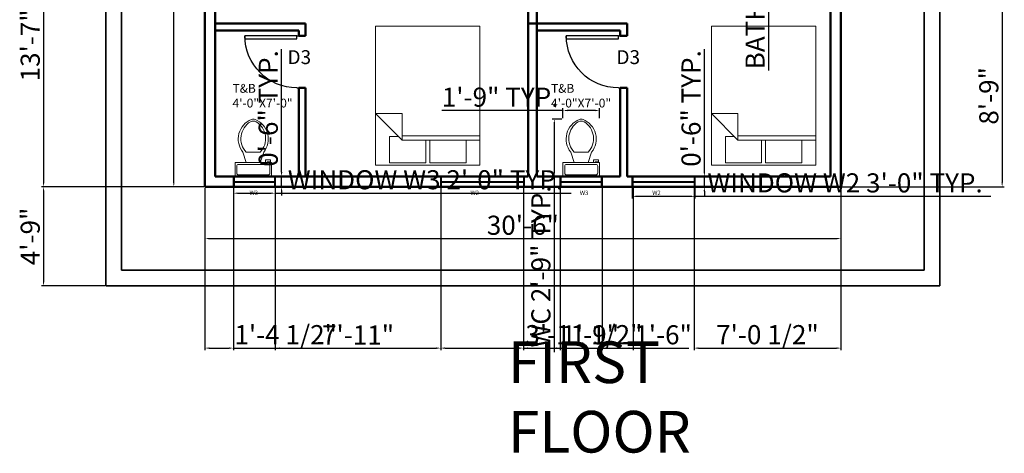
# Model space of a CAD drawing. Units: inches. Extents: x 2299 to 4423, y 1066 to 1805.
# Tile 4 of 7: x 3069 to 3636, y 1066 to 1315. Entities that reach past the tile are written whole.
import ezdxf

# ---------------------------------------------------------------- set-up
doc = ezdxf.new("R2010")
doc.units = ezdxf.units.IN
for name, color, linetype, lineweight in [('A-ANNO-DIMS', 2, 'Continuous', 18), ('A-ANNO-TEXT', 1, 'Continuous', 25), ('A-AREA-IDEN', 1, 'Continuous', 25), ('A-DOOR', 5, 'Continuous', 25), ('A-FURN', 8, 'Continuous', 18), ('A-GLAZ', 3, 'Continuous', 25), ('A-WALL', 7, 'Continuous', 50), ('C-PROP', 7, 'Continuous', 35)]:
    doc.layers.add(name, color=color, linetype=linetype, lineweight=lineweight)
doc.styles.get("Standard").update_dxf_attribs({"font": 'arial.ttf'})
doc.dimstyles.new('ISO-25', dxfattribs={"dimtxt": 11, "dimasz": 2.5, "dimexe": 1.25, "dimexo": 0.625, "dimtad": 1, "dimlunit": 4, "dimtxsty": 'Standard', "dimcen": 2.5, "dimadec": 0, "dimazin": 0, "dimtfac": 1, "dimtmove": 0, "dimatfit": 3, "dimfxl": 1, "dimarcsym": 0})

# ---------------------------------------------------------------- blocks, each defined once
blk = doc.blocks.new('*U2')
for p, q in [((0, 0), (0, -5)), ((30, 0), (30, -5))]:
    blk.add_line(p, q)
blk.add_lwpolyline([(0, 0), (0, 30), (1.75, 30), (1.75, 0)], close=True)
blk.add_arc((0, 0), 30, 0, 90)
blk = doc.blocks.new('Bed - Queen')
for p, q in [((0, -80.00003), (0, 0)), ((0, 0), (59.99999, 0)), ((59.99999, 0), (59.99999, -80.00003)), ((7.99999, -1.2), (28.79998, -1.2)), ((7.99999, -14.4), (7.99999, -1.2)), ((28.79998, -1.2), (28.79998, -14.4)), ((31.19999, -1.2), (51.99999, -1.2)), ((31.19999, -14.4), (31.19999, -1.2)), ((51.99999, -1.2), (51.99999, -16.4)), ((0, -14.4), (44.8, -14.4)), ((44.8, -16.8), (0, -16.8)), ((59.99999, -29.6), (44.8, -14.4)), ((44.8, -14.4), (44.8, -29.6)), ((51.99999, -16.4), (46.79936, -16.4)), ((44.8, -29.6), (59.99999, -29.6)), ((59.99999, -80.00003), (0, -80.00003))]:
    blk.add_line(p, q)
blk = doc.blocks.new('Toilet - top')
for p, q in [((9.5, -6), (9.5, -2)), ((-10, -8.5), (-8, -8.5)), ((-10, -9.5), (-10, -8.5)), ((-7, -9.5), (-10, -9.5)), ((-8, -8.5), (-8, -8)), ((-7, -8), (-7, -9.5)), ((-4, -8), (-6, -14)), ((4, -8), (6, -14)), ((4, -14), (-4, -14))]:
    blk.add_line(p, q)
blk.add_lwpolyline([(10.5, -8), (10.5, 0), (-10.5, 0), (-10.5, -8)], close=True)
for points in [[(-9.5, -2), (-9.5, -6)], [(8.5, -1), (-8.5, -1)], [(-8.5, -7), (8.5, -7)]]:
    blk.add_lwpolyline(points)
for centre, radius, start, end in [((-8.62, -1.88), 0.884, 81.8699, 188.1301), ((8.62, -1.88), 0.884, 351.8699, 98.1301), ((-8.62, -6.12), 0.884, 171.8699, 278.1301), ((8.62, -6.12), 0.884, 261.8699, 8.1301), ((3.52, -21.58), 12.17, 141.4691, 247.9714), ((4.2, -21.82), 11.33, 136.3677, 238.9468), ((-3.52, -21.58), 12.17, 292.0284, 38.5307), ((-4.2, -21.82), 11.33, 301.053, 43.6321), ((0, -27.88), 4, 245.7318, 294.2682), ((0, -29), 4, 254.8605, 285.1395)]:
    blk.add_arc(centre, radius, start, end)
blk = doc.blocks.new('*D24')
at = {"layer": 'A-ANNO-DIMS', "color": 0, "lineweight": -2, "transparency": 16777216}
for p, q in [((3175.75, 1218.32), (3175.75, 1187.97)), ((3541.75, 1218.32), (3541.75, 1187.97)), ((3178.25, 1189.22), (3539.25, 1189.22))]:
    blk.add_line(p, q, dxfattribs=at)
at = {"layer": 'A-ANNO-DIMS', "color": 0, "transparency": 16777216}
for points in [[(3178.25, 1189.63), (3178.25, 1188.8), (3175.75, 1189.22)], [(3539.25, 1189.63), (3539.25, 1188.8), (3541.75, 1189.22)]]:
    blk.add_solid(points, dxfattribs=at)
at = {"layer": 'Defpoints', "color": 0, "transparency": 16777216}
for p in [(3175.75, 1218.95), (3541.75, 1218.95), (3541.75, 1189.22)]:
    blk.add_point(p, dxfattribs=at)
at = {"layer": 'A-ANNO-DIMS', "color": 0, "transparency": 16777216, "insert": (3358.75, 1195.46), "char_height": 11, "attachment_point": 5}
blk.add_mtext('30\'-6"', dxfattribs=at)
blk = doc.blocks.new('*D25')
at = {"layer": 'A-ANNO-DIMS', "color": 0, "lineweight": -2, "transparency": 16777216}
for p, q in [((3175.12, 1680.95), (3156.64, 1680.95)), ((3157.89, 1221.45), (3157.89, 1678.45)), ((3175.12, 1218.95), (3156.64, 1218.95))]:
    blk.add_line(p, q, dxfattribs=at)
at = {"layer": 'A-ANNO-DIMS', "color": 0, "transparency": 16777216}
for points in [[(3157.47, 1678.45), (3158.3, 1678.45), (3157.89, 1680.95)], [(3157.47, 1221.45), (3158.3, 1221.45), (3157.89, 1218.95)]]:
    blk.add_solid(points, dxfattribs=at)
at = {"layer": 'Defpoints', "color": 0, "transparency": 16777216}
for p in [(3157.89, 1680.95), (3175.75, 1680.95), (3175.75, 1218.95)]:
    blk.add_point(p, dxfattribs=at)
at = {"layer": 'A-ANNO-DIMS', "color": 0, "transparency": 16777216, "insert": (3151.64, 1449.95), "char_height": 11, "attachment_point": 5, "rotation": 90}
blk.add_mtext('38\'-6"', dxfattribs=at)
blk = doc.blocks.new('WIN-1200')
for p, q in [((0, 0), (0, 48.07)), ((0, 48.07), (6, 48.07)), ((0, 47.57), (6, 47.57)), ((2.8, 47.57), (2.8, 0.5)), ((3.2, 47.57), (3.2, 0.5)), ((6, 48.07), (6, 0)), ((6, 0.5), (0, 0.5)), ((6, 0), (0, 0))]:
    blk.add_line(p, q)
blk = doc.blocks.new('WIN-600')
for p, q in [((0, 6), (24.07, 6)), ((0, 0), (0, 6)), ((0.5, 0), (0.5, 6)), ((23.57, 6), (23.57, 0)), ((24.07, 6), (24.07, 0)), ((24.07, 0), (0, 0)), ((0.5, 3.2), (23.57, 3.2)), ((0.5, 2.8), (23.57, 2.8))]:
    blk.add_line(p, q)
blk = doc.blocks.new('WIN-900')
for p, q in [((0, 6), (36.07, 6)), ((0, 0), (0, 6)), ((0.5, 0), (0.5, 6)), ((35.57, 6), (35.57, 0)), ((36.07, 6), (36.07, 0)), ((36.07, 0), (0, 0)), ((0.5, 3.2), (35.57, 3.2)), ((0.5, 2.8), (35.57, 2.8))]:
    blk.add_line(p, q)
blk = doc.blocks.new('*D44')
at = {"layer": 'A-ANNO-DIMS', "color": 0, "lineweight": -2, "transparency": 16777216}
for p, q in [((3192.23, 1218.32), (3192.23, 1214.08)), ((3216.3, 1218.32), (3216.3, 1214.08)), ((3194.73, 1215.33), (3213.8, 1215.33)), ((3216.3, 1215.33), (3386.57, 1215.33))]:
    blk.add_line(p, q, dxfattribs=at)
at = {"layer": 'A-ANNO-DIMS', "color": 0, "transparency": 16777216}
for points in [[(3194.73, 1215.75), (3194.73, 1214.92), (3192.23, 1215.33)], [(3213.8, 1215.75), (3213.8, 1214.92), (3216.3, 1215.33)]]:
    blk.add_solid(points, dxfattribs=at)
at = {"layer": 'Defpoints', "color": 0, "transparency": 16777216}
for p in [(3192.23, 1218.95), (3216.3, 1218.95), (3216.3, 1215.33)]:
    blk.add_point(p, dxfattribs=at)
at = {"layer": 'A-ANNO-DIMS', "color": 0, "transparency": 16777216, "insert": (3302.69, 1221.65), "char_height": 11, "attachment_point": 5}
blk.add_mtext('WINDOW W3 2\'-0" TYP.', dxfattribs=at)
blk = doc.blocks.new('*D45')
at = {"layer": 'A-ANNO-DIMS', "color": 0, "lineweight": -2, "transparency": 16777216}
for p, q in [((3219.92, 1227.45), (3219.92, 1298.25)), ((3216.93, 1224.95), (3221.17, 1224.95)), ((3219.92, 1218.95), (3219.92, 1224.95)), ((3216.93, 1218.95), (3221.17, 1218.95)), ((3219.92, 1216.45), (3219.92, 1213.95))]:
    blk.add_line(p, q, dxfattribs=at)
at = {"layer": 'A-ANNO-DIMS', "color": 0, "transparency": 16777216}
for points in [[(3219.5, 1227.45), (3220.33, 1227.45), (3219.92, 1224.95)], [(3219.5, 1216.45), (3220.33, 1216.45), (3219.92, 1218.95)]]:
    blk.add_solid(points, dxfattribs=at)
at = {"layer": 'Defpoints', "color": 0, "transparency": 16777216}
for p in [(3216.3, 1224.95), (3219.92, 1224.95), (3216.3, 1218.95)]:
    blk.add_point(p, dxfattribs=at)
at = {"layer": 'A-ANNO-DIMS', "color": 0, "transparency": 16777216, "insert": (3213.67, 1264.1), "char_height": 11, "attachment_point": 5, "rotation": 90}
blk.add_mtext('0\'-6" TYP.', dxfattribs=at)
blk = doc.blocks.new('*D46')
at = {"layer": 'A-ANNO-DIMS', "color": 0, "lineweight": -2, "transparency": 16777216}
for p, q in [((3381.19, 1257.99), (3375.61, 1257.99)), ((3376.86, 1255.49), (3376.86, 1227.45)), ((3381.19, 1224.95), (3375.61, 1224.95)), ((3376.86, 1224.95), (3376.86, 1123.82))]:
    blk.add_line(p, q, dxfattribs=at)
at = {"layer": 'A-ANNO-DIMS', "color": 0, "transparency": 16777216}
for points in [[(3376.44, 1255.49), (3377.28, 1255.49), (3376.86, 1257.99)], [(3376.44, 1227.45), (3377.28, 1227.45), (3376.86, 1224.95)]]:
    blk.add_solid(points, dxfattribs=at)
at = {"layer": 'Defpoints', "color": 0, "transparency": 16777216}
for p in [(3381.82, 1257.99), (3376.86, 1224.95), (3381.82, 1224.95)]:
    blk.add_point(p, dxfattribs=at)
at = {"layer": 'A-ANNO-DIMS', "color": 0, "transparency": 16777216, "insert": (3370.55, 1173.13), "char_height": 11, "attachment_point": 5, "rotation": 90}
blk.add_mtext('WC 2\'-9" TYP.', dxfattribs=at)
blk = doc.blocks.new('*D47')
at = {"layer": 'A-ANNO-DIMS', "color": 0, "lineweight": -2, "transparency": 16777216}
for p, q in [((3381.82, 1258.62), (3381.82, 1264.2)), ((3402.82, 1258.62), (3402.82, 1264.2)), ((3381.82, 1262.95), (3312.05, 1262.95)), ((3400.32, 1262.95), (3384.32, 1262.95))]:
    blk.add_line(p, q, dxfattribs=at)
at = {"layer": 'A-ANNO-DIMS', "color": 0, "transparency": 16777216}
for points in [[(3384.32, 1263.37), (3384.32, 1262.53), (3381.82, 1262.95)], [(3400.32, 1263.37), (3400.32, 1262.53), (3402.82, 1262.95)]]:
    blk.add_solid(points, dxfattribs=at)
at = {"layer": 'Defpoints', "color": 0, "transparency": 16777216}
for p in [(3381.82, 1262.95), (3381.82, 1257.99), (3402.82, 1257.99)]:
    blk.add_point(p, dxfattribs=at)
at = {"layer": 'A-ANNO-DIMS', "color": 0, "transparency": 16777216, "insert": (3345.68, 1269.19), "char_height": 11, "attachment_point": 5}
blk.add_mtext('1\'-9" TYP.', dxfattribs=at)
blk = doc.blocks.new('*D50')
at = {"layer": 'A-ANNO-DIMS', "color": 0, "lineweight": -2, "transparency": 16777216}
for p, q in [((3421.72, 1218.32), (3421.72, 1212.28)), ((3457.79, 1218.32), (3457.79, 1212.28)), ((3424.22, 1213.53), (3455.29, 1213.53)), ((3457.79, 1213.53), (3628.06, 1213.53))]:
    blk.add_line(p, q, dxfattribs=at)
at = {"layer": 'A-ANNO-DIMS', "color": 0, "transparency": 16777216}
for points in [[(3424.22, 1213.95), (3424.22, 1213.12), (3421.72, 1213.53)], [(3455.29, 1213.95), (3455.29, 1213.12), (3457.79, 1213.53)]]:
    blk.add_solid(points, dxfattribs=at)
at = {"layer": 'Defpoints', "color": 0, "transparency": 16777216}
for p in [(3421.72, 1218.95), (3457.79, 1218.95), (3457.79, 1213.53)]:
    blk.add_point(p, dxfattribs=at)
at = {"layer": 'A-ANNO-DIMS', "color": 0, "transparency": 16777216, "insert": (3544.17, 1219.85), "char_height": 11, "attachment_point": 5}
blk.add_mtext('WINDOW W2 3\'-0" TYP.', dxfattribs=at)
blk = doc.blocks.new('*D51')
at = {"layer": 'A-ANNO-DIMS', "color": 0, "lineweight": -2, "transparency": 16777216}
for p, q in [((3463.2, 1227.45), (3463.2, 1298.25)), ((3458.42, 1224.95), (3464.45, 1224.95)), ((3463.2, 1218.95), (3463.2, 1224.95)), ((3458.42, 1218.95), (3464.45, 1218.95)), ((3463.2, 1216.45), (3463.2, 1213.95))]:
    blk.add_line(p, q, dxfattribs=at)
at = {"layer": 'A-ANNO-DIMS', "color": 0, "transparency": 16777216}
for points in [[(3462.79, 1227.45), (3463.62, 1227.45), (3463.2, 1224.95)], [(3462.79, 1216.45), (3463.62, 1216.45), (3463.2, 1218.95)]]:
    blk.add_solid(points, dxfattribs=at)
at = {"layer": 'Defpoints', "color": 0, "transparency": 16777216}
for p in [(3457.79, 1224.95), (3463.2, 1224.95), (3457.79, 1218.95)]:
    blk.add_point(p, dxfattribs=at)
at = {"layer": 'A-ANNO-DIMS', "color": 0, "transparency": 16777216, "insert": (3456.96, 1264.1), "char_height": 11, "attachment_point": 5, "rotation": 90}
blk.add_mtext('0\'-6" TYP.', dxfattribs=at)
blk = doc.blocks.new('*D58')
at = {"layer": 'A-ANNO-DIMS', "color": 0, "lineweight": -2, "transparency": 16777216}
for p, q in [((3506.06, 1467.99), (3498.88, 1467.99)), ((3500.13, 1465.49), (3500.13, 1426.78)), ((3506.06, 1424.28), (3498.88, 1424.28)), ((3500.13, 1424.28), (3500.13, 1285.89))]:
    blk.add_line(p, q, dxfattribs=at)
at = {"layer": 'A-ANNO-DIMS', "color": 0, "transparency": 16777216}
for points in [[(3499.71, 1465.49), (3500.55, 1465.49), (3500.13, 1467.99)], [(3499.71, 1426.78), (3500.55, 1426.78), (3500.13, 1424.28)]]:
    blk.add_solid(points, dxfattribs=at)
at = {"layer": 'Defpoints', "color": 0, "transparency": 16777216}
for p in [(3506.69, 1467.99), (3500.13, 1424.28), (3506.69, 1424.28)]:
    blk.add_point(p, dxfattribs=at)
at = {"layer": 'A-ANNO-DIMS', "color": 0, "transparency": 16777216, "insert": (3493.81, 1353.83), "char_height": 11, "attachment_point": 5, "rotation": 90}
blk.add_mtext('BATH TUB 3\'-7 1/2"', dxfattribs=at)
blk = doc.blocks.new('*D102')
at = {"layer": 'A-ANNO-DIMS', "color": 0, "lineweight": -2, "transparency": 16777216}
for p, q in [((3181.12, 1381.95), (3081.7, 1381.95)), ((3082.95, 1379.45), (3082.95, 1221.45)), ((3175.12, 1218.95), (3081.7, 1218.95))]:
    blk.add_line(p, q, dxfattribs=at)
at = {"layer": 'A-ANNO-DIMS', "color": 0, "transparency": 16777216}
for points in [[(3082.53, 1379.45), (3083.37, 1379.45), (3082.95, 1381.95)], [(3082.53, 1221.45), (3083.37, 1221.45), (3082.95, 1218.95)]]:
    blk.add_solid(points, dxfattribs=at)
at = {"layer": 'Defpoints', "color": 0, "transparency": 16777216}
for p in [(3181.75, 1381.95), (3082.95, 1218.95), (3175.75, 1218.95)]:
    blk.add_point(p, dxfattribs=at)
at = {"layer": 'A-ANNO-DIMS', "color": 0, "transparency": 16777216, "insert": (3076.7, 1300.45), "char_height": 11, "attachment_point": 5, "rotation": 90}
blk.add_mtext('13\'-7"', dxfattribs=at)
blk = doc.blocks.new('*D103')
at = {"layer": 'A-ANNO-DIMS', "color": 0, "lineweight": -2, "transparency": 16777216}
for p, q in [((3175.12, 1218.95), (3081.7, 1218.95)), ((3082.95, 1216.45), (3082.95, 1164.45)), ((3118.12, 1161.95), (3081.7, 1161.95))]:
    blk.add_line(p, q, dxfattribs=at)
at = {"layer": 'A-ANNO-DIMS', "color": 0, "transparency": 16777216}
for points in [[(3082.53, 1216.45), (3083.37, 1216.45), (3082.95, 1218.95)], [(3082.53, 1164.45), (3083.37, 1164.45), (3082.95, 1161.95)]]:
    blk.add_solid(points, dxfattribs=at)
at = {"layer": 'Defpoints', "color": 0, "transparency": 16777216}
for p in [(3175.75, 1218.95), (3082.95, 1161.95), (3118.75, 1161.95)]:
    blk.add_point(p, dxfattribs=at)
at = {"layer": 'A-ANNO-DIMS', "color": 0, "transparency": 16777216, "insert": (3076.71, 1190.45), "char_height": 11, "attachment_point": 5, "rotation": 90}
blk.add_mtext('4\'-9"', dxfattribs=at)
blk = doc.blocks.new('*D108')
at = {"layer": 'A-ANNO-DIMS', "color": 0, "lineweight": -2, "transparency": 16777216}
for p, q in [((3542.37, 1323.79), (3635.8, 1323.79)), ((3634.55, 1321.29), (3634.55, 1221.45)), ((3542.37, 1218.95), (3635.8, 1218.95))]:
    blk.add_line(p, q, dxfattribs=at)
at = {"layer": 'A-ANNO-DIMS', "color": 0, "transparency": 16777216}
for points in [[(3634.13, 1321.29), (3634.97, 1321.29), (3634.55, 1323.79)], [(3634.13, 1221.45), (3634.97, 1221.45), (3634.55, 1218.95)]]:
    blk.add_solid(points, dxfattribs=at)
at = {"layer": 'Defpoints', "color": 0, "transparency": 16777216}
for p in [(3541.75, 1323.79), (3541.75, 1218.95), (3634.55, 1218.95)]:
    blk.add_point(p, dxfattribs=at)
at = {"layer": 'A-ANNO-DIMS', "color": 0, "transparency": 16777216, "insert": (3628.31, 1271.37), "char_height": 11, "attachment_point": 5, "rotation": 90}
blk.add_mtext('8\'-9"', dxfattribs=at)
blk = doc.blocks.new('*D109')
at = {"layer": 'A-ANNO-DIMS', "color": 0, "lineweight": -2, "transparency": 16777216}
for p, q in [((3175.75, 1218.32), (3175.75, 1124.9)), ((3192.23, 1218.32), (3192.23, 1124.9)), ((3178.25, 1126.15), (3189.73, 1126.15)), ((3192.23, 1126.15), (3249.82, 1126.15))]:
    blk.add_line(p, q, dxfattribs=at)
at = {"layer": 'A-ANNO-DIMS', "color": 0, "transparency": 16777216}
for points in [[(3178.25, 1126.56), (3178.25, 1125.73), (3175.75, 1126.15)], [(3189.73, 1126.56), (3189.73, 1125.73), (3192.23, 1126.15)]]:
    blk.add_solid(points, dxfattribs=at)
at = {"layer": 'Defpoints', "color": 0, "transparency": 16777216}
for p in [(3175.75, 1218.95), (3192.23, 1218.95), (3192.23, 1126.15)]:
    blk.add_point(p, dxfattribs=at)
at = {"layer": 'A-ANNO-DIMS', "color": 0, "transparency": 16777216, "insert": (3222.28, 1132.46), "char_height": 11, "attachment_point": 5}
blk.add_mtext('1\'-4 1/2"', dxfattribs=at)
blk = doc.blocks.new('*D110')
at = {"layer": 'A-ANNO-DIMS', "color": 0, "lineweight": -2, "transparency": 16777216}
for p, q in [((3216.3, 1218.32), (3216.3, 1124.9)), ((3311.49, 1218.32), (3311.49, 1124.9)), ((3218.8, 1126.15), (3308.99, 1126.15))]:
    blk.add_line(p, q, dxfattribs=at)
at = {"layer": 'A-ANNO-DIMS', "color": 0, "transparency": 16777216}
for points in [[(3218.8, 1126.56), (3218.8, 1125.73), (3216.3, 1126.15)], [(3308.99, 1126.56), (3308.99, 1125.73), (3311.49, 1126.15)]]:
    blk.add_solid(points, dxfattribs=at)
at = {"layer": 'Defpoints', "color": 0, "transparency": 16777216}
for p in [(3216.3, 1218.95), (3311.49, 1218.95), (3311.49, 1126.15)]:
    blk.add_point(p, dxfattribs=at)
at = {"layer": 'A-ANNO-DIMS', "color": 0, "transparency": 16777216, "insert": (3263.9, 1132.29), "char_height": 11, "attachment_point": 5}
blk.add_mtext('7\'-11"', dxfattribs=at)
blk = doc.blocks.new('*D111')
at = {"layer": 'A-ANNO-DIMS', "color": 0, "lineweight": -2, "transparency": 16777216}
for p, q in [((3311.49, 1218.32), (3311.49, 1124.9)), ((3359.06, 1218.32), (3359.06, 1124.9)), ((3313.99, 1126.15), (3356.56, 1126.15)), ((3359.06, 1126.15), (3426.22, 1126.15))]:
    blk.add_line(p, q, dxfattribs=at)
at = {"layer": 'A-ANNO-DIMS', "color": 0, "transparency": 16777216}
for points in [[(3313.99, 1126.56), (3313.99, 1125.73), (3311.49, 1126.15)], [(3356.56, 1126.56), (3356.56, 1125.73), (3359.06, 1126.15)]]:
    blk.add_solid(points, dxfattribs=at)
at = {"layer": 'Defpoints', "color": 0, "transparency": 16777216}
for p in [(3311.49, 1218.95), (3359.06, 1218.95), (3359.06, 1126.15)]:
    blk.add_point(p, dxfattribs=at)
at = {"layer": 'A-ANNO-DIMS', "color": 0, "transparency": 16777216, "insert": (3393.89, 1132.46), "char_height": 11, "attachment_point": 5}
blk.add_mtext('3\'-11 1/2"', dxfattribs=at)
blk = doc.blocks.new('*D112')
at = {"layer": 'A-ANNO-DIMS', "color": 0, "lineweight": -2, "transparency": 16777216}
for p, q in [((3359.06, 1218.32), (3359.06, 1124.9)), ((3380.28, 1218.32), (3380.28, 1124.9)), ((3361.56, 1126.15), (3377.78, 1126.15)), ((3380.28, 1126.15), (3412.24, 1126.15))]:
    blk.add_line(p, q, dxfattribs=at)
at = {"layer": 'A-ANNO-DIMS', "color": 0, "transparency": 16777216}
for points in [[(3361.56, 1126.56), (3361.56, 1125.73), (3359.06, 1126.15)], [(3377.78, 1126.56), (3377.78, 1125.73), (3380.28, 1126.15)]]:
    blk.add_solid(points, dxfattribs=at)
at = {"layer": 'Defpoints', "color": 0, "transparency": 16777216}
for p in [(3359.06, 1218.95), (3380.28, 1218.95), (3380.28, 1126.15)]:
    blk.add_point(p, dxfattribs=at)
at = {"layer": 'A-ANNO-DIMS', "color": 0, "transparency": 16777216, "insert": (3397.51, 1132.39), "char_height": 11, "attachment_point": 5}
blk.add_mtext('1\'-9"', dxfattribs=at)
blk = doc.blocks.new('*D113')
at = {"layer": 'A-ANNO-DIMS', "color": 0, "lineweight": -2, "transparency": 16777216}
for p, q in [((3404.35, 1218.32), (3404.35, 1124.9)), ((3422.22, 1218.32), (3422.22, 1124.9)), ((3406.85, 1126.15), (3419.72, 1126.15)), ((3422.22, 1126.15), (3454.18, 1126.15))]:
    blk.add_line(p, q, dxfattribs=at)
at = {"layer": 'A-ANNO-DIMS', "color": 0, "transparency": 16777216}
for points in [[(3406.85, 1126.56), (3406.85, 1125.73), (3404.35, 1126.15)], [(3419.72, 1126.56), (3419.72, 1125.73), (3422.22, 1126.15)]]:
    blk.add_solid(points, dxfattribs=at)
at = {"layer": 'Defpoints', "color": 0, "transparency": 16777216}
for p in [(3404.35, 1218.95), (3422.22, 1218.95), (3422.22, 1126.15)]:
    blk.add_point(p, dxfattribs=at)
at = {"layer": 'A-ANNO-DIMS', "color": 0, "transparency": 16777216, "insert": (3439.45, 1132.39), "char_height": 11, "attachment_point": 5}
blk.add_mtext('1\'-6"', dxfattribs=at)
blk = doc.blocks.new('*D114')
at = {"layer": 'A-ANNO-DIMS', "color": 0, "lineweight": -2, "transparency": 16777216}
for p, q in [((3457.29, 1218.32), (3457.29, 1124.9)), ((3541.75, 1218.32), (3541.75, 1124.9)), ((3459.79, 1126.15), (3539.25, 1126.15))]:
    blk.add_line(p, q, dxfattribs=at)
at = {"layer": 'A-ANNO-DIMS', "color": 0, "transparency": 16777216}
for points in [[(3459.79, 1126.56), (3459.79, 1125.73), (3457.29, 1126.15)], [(3539.25, 1126.56), (3539.25, 1125.73), (3541.75, 1126.15)]]:
    blk.add_solid(points, dxfattribs=at)
at = {"layer": 'Defpoints', "color": 0, "transparency": 16777216}
for p in [(3457.29, 1218.95), (3541.75, 1218.95), (3541.75, 1126.15)]:
    blk.add_point(p, dxfattribs=at)
at = {"layer": 'A-ANNO-DIMS', "color": 0, "transparency": 16777216, "insert": (3499.52, 1132.46), "char_height": 11, "attachment_point": 5}
blk.add_mtext('7\'-0 1/2"', dxfattribs=at)

msp = doc.modelspace()

# ---------------------------------------------------------------- linework, layer by layer
at = {"layer": 'A-WALL'}
for p, q in [((3175.749, 1218.945), (3175.749, 1680.945)), ((3181.749, 1224.945), (3181.749, 1376.945)), ((3361.749, 1224.945), (3361.749, 1381.945)), ((3366.749, 1224.945), (3366.749, 1376.945)), ((3535.749, 1224.945), (3535.749, 1349.945)), ((3541.749, 1218.945), (3541.749, 1344.945)), ((3233.749, 1312.945), (3181.749, 1312.945)), ((3229.749, 1308.945), (3181.749, 1308.945)), ((3229.749, 1308.945), (3229.749, 1305.945)), ((3229.749, 1305.945), (3229.749, 1308.945)), ((3233.749, 1305.945), (3233.749, 1312.945)), ((3418.749, 1312.945), (3361.749, 1312.945)), ((3414.749, 1308.945), (3366.749, 1308.945)), ((3414.749, 1308.945), (3414.749, 1305.945)), ((3414.749, 1305.945), (3414.749, 1308.945)), ((3418.749, 1305.945), (3418.749, 1312.945)), ((3229.749, 1305.945), (3233.749, 1305.945)), ((3414.749, 1305.945), (3418.749, 1305.945)), ((3229.749, 1224.945), (3229.749, 1275.945)), ((3233.749, 1275.945), (3229.749, 1275.945)), ((3233.749, 1224.945), (3233.749, 1275.945)), ((3414.749, 1224.945), (3414.749, 1275.945)), ((3418.749, 1275.945), (3414.749, 1275.945)), ((3418.749, 1224.945), (3418.749, 1275.945)), ((3361.749, 1224.945), (3181.749, 1224.945)), ((3410.749, 1224.945), (3366.749, 1224.945)), ((3410.749, 1224.945), (3414.749, 1224.945)), ((3418.749, 1224.945), (3535.749, 1224.945)), ((3415.749, 1218.945), (3175.749, 1218.945)), ((3415.749, 1218.945), (3541.749, 1218.945))]:
    msp.add_line(p, q, dxfattribs=at)
at = {"layer": 'C-PROP'}
for p, q in [((3118.749, 1161.945), (3118.749, 1737.945)), ((3598.749, 1737.945), (3598.749, 1161.945)), ((3127.749, 1170.945), (3127.749, 1728.945)), ((3589.749, 1728.945), (3589.749, 1170.945)), ((3589.749, 1170.945), (3127.749, 1170.945)), ((3598.749, 1161.945), (3118.749, 1161.945))]:
    msp.add_line(p, q, dxfattribs=at)

# ---------------------------------------------------------------- block references
at = {"layer": 'A-DOOR', "xscale": -1, "rotation": 90}
for p in [(3228.749, 1305.945), (3413.749, 1305.945)]:
    msp.add_blockref('*U2', p, dxfattribs=at)
at = {"layer": 'A-FURN'}
for name, p, rotation in [('Bed - Queen', (3334.043, 1231.522), 179.9999999999998), ('Bed - Queen', (3527.273, 1231.522), 179.9999999999998), ('Toilet - top', (3203.62, 1224.945), 180), ('Toilet - top', (3392.317, 1224.945), 180)]:
    msp.add_blockref(name, p, dxfattribs=dict(at, rotation=rotation))
at = {"layer": 'A-GLAZ'}
for name, p in [('WIN-600', (3192.233, 1218.945)), ('WIN-600', (3380.282, 1218.945)), ('WIN-900', (3421.72, 1218.945))]:
    msp.add_blockref(name, p, dxfattribs=at)
at = {"layer": 'A-GLAZ', "rotation": 89.99999999999973}
msp.add_blockref('WIN-1200', (3359.563, 1218.945), dxfattribs=at)

# ---------------------------------------------------------------- texts
at = {"layer": 'A-ANNO-TEXT', "attachment_point": 1}
for s, width, gutter_width, insert, char_height in [('D3', 1.11117, 12.5, (3223.344, 1297.671), 8), ('D3', 1.11117, 12.5, (3412.638, 1297.671), 8), ('FIRST\\PFLOOR', 684.73543, 351.786, (3350.163, 1130.01), 24)]:
    msp.add_mtext_dynamic_manual_height_columns(s, width=width, gutter_width=gutter_width, heights=[0], dxfattribs=dict(at, insert=insert, char_height=char_height))
at = {"layer": 'A-ANNO-TEXT', "char_height": 2.5, "attachment_point": 1}
for s, insert in [('W3', (3201.458, 1216.805)), ('W2', (3328.604, 1216.805)), ('W3', (3391.551, 1216.805)), ('W2', (3433.203, 1216.805))]:
    msp.add_mtext(s, dxfattribs=dict(at, insert=insert))
at = {"layer": 'A-AREA-IDEN', "char_height": 5.07992, "attachment_point": 1}
for insert in [(3191.657, 1278.226), (3374.948, 1278.226)]:
    msp.add_mtext_dynamic_manual_height_columns('T&B\\P4\'-0"X7\'-0"', width=2.46662, gutter_width=25.4, heights=[0], dxfattribs=dict(at, insert=insert))

# ---------------------------------------------------------------- dimensions: what is measured, and where the dimension line sits
at = {"layer": 'A-ANNO-DIMS'}
for base, p1, p2, override, picture, middle in [((3157.885, 1680.945), (3175.749, 1218.945), (3175.749, 1680.945), {"dimclrd": 0, "dimclre": 0, "dimclrt": 0}, '*D25', (3151.64, 1449.945)), ((3082.949, 1218.945), (3181.749, 1381.945), (3175.749, 1218.945), {"dimdec": 1, "dimlfac": 1, "dimrnd": 0, "dimzin": 1, "dimdsep": 46, "dimlunit": 4, "dimfrac": 2}, '*D102', (3076.704, 1300.445)), ((3634.549, 1218.945), (3541.749, 1323.793), (3541.749, 1218.945), {"dimdec": 1, "dimlfac": 1, "dimrnd": 0, "dimzin": 1, "dimdsep": 46, "dimlunit": 4, "dimfrac": 2}, '*D108', (3628.308, 1271.369)), ((3082.949, 1161.945), (3175.749, 1218.945), (3118.749, 1161.945), {"dimdec": 1, "dimlfac": 1, "dimrnd": 0, "dimzin": 1, "dimdsep": 46, "dimlunit": 4, "dimfrac": 2}, '*D103', (3076.708, 1190.445))]:
    dim = msp.add_linear_dim(base=base, p1=p1, p2=p2, angle=90, dimstyle='ISO-25', override=override, dxfattribs=at)
    dim.commit()
    dim.dimension.update_dxf_attribs({"geometry": picture, "text_midpoint": middle})
for base, p1, p2, angle, text, picture, middle in [((3500.129, 1424.28), (3506.686, 1467.993), (3506.686, 1424.28), 270, 'BATH TUB <>', '*D58', (3493.812, 1353.834)), ((3219.915, 1224.945), (3216.305, 1218.945), (3216.305, 1224.945), 90, '<> TYP.', '*D45', (3213.674, 1264.096)), ((3463.202, 1224.945), (3457.791, 1218.945), (3457.791, 1224.945), 90, '<> TYP.', '*D51', (3456.961, 1264.096)), ((3381.817, 1262.949), (3402.817, 1257.992), (3381.817, 1257.992), 180, '<> TYP.', '*D47', (3345.685, 1269.19)), ((3376.861, 1224.945), (3381.817, 1257.992), (3381.817, 1224.945), 270, 'WC <> TYP.', '*D46', (3370.548, 1173.134))]:
    dim = msp.add_linear_dim(base=base, p1=p1, p2=p2, angle=angle, text=text, dimstyle='ISO-25', override={"dimdec": 1, "dimrnd": 0, "dimzin": 1, "dimlunit": 4, "dimfrac": 2}, dxfattribs=at)
    dim.commit()
    dim.dimension.update_dxf_attribs({"geometry": picture, "text_midpoint": middle})
for base, p1, p2, text, picture, middle in [((3216.305, 1215.335), (3192.234, 1218.945), (3216.305, 1218.945), 'WINDOW W3 <> TYP.', '*D44', (3302.687, 1221.655)), ((3457.791, 1213.535), (3421.72, 1218.945), (3457.791, 1218.945), 'WINDOW W2 <> TYP.', '*D50', (3544.174, 1219.855))]:
    dim = msp.add_linear_dim(base=base, p1=p1, p2=p2, text=text, dimstyle='ISO-25', override={"dimdec": 1, "dimrnd": 0, "dimzin": 1, "dimlunit": 4, "dimfrac": 2}, dxfattribs=at)
    dim.commit()
    dim.dimension.update_dxf_attribs({"geometry": picture, "text_midpoint": middle})
for base, p1, p2, override, picture, middle in [((3541.749, 1189.218), (3175.749, 1218.945), (3541.749, 1218.945), {"dimclrd": 0, "dimclre": 0, "dimclrt": 0}, '*D24', (3358.749, 1195.463)), ((3192.234, 1126.145), (3175.749, 1218.945), (3192.234, 1218.945), {"dimdec": 1, "dimlfac": 1, "dimrnd": 0, "dimzin": 1, "dimdsep": 46, "dimlunit": 4, "dimfrac": 2}, '*D109', (3222.277, 1132.458)), ((3311.492, 1126.145), (3216.305, 1218.945), (3311.492, 1218.945), {"dimdec": 1, "dimlfac": 1, "dimrnd": 0, "dimzin": 1, "dimdsep": 46, "dimlunit": 4, "dimfrac": 2}, '*D110', (3263.899, 1132.293)), ((3359.063, 1126.145), (3311.492, 1218.945), (3359.063, 1218.945), {"dimdec": 1, "dimlfac": 1, "dimrnd": 0, "dimzin": 1, "dimdsep": 46, "dimlunit": 4, "dimfrac": 2}, '*D111', (3393.894, 1132.462)), ((3380.282, 1126.145), (3359.063, 1218.945), (3380.282, 1218.945), {"dimdec": 1, "dimlfac": 1, "dimrnd": 0, "dimzin": 1, "dimdsep": 46, "dimlunit": 4, "dimfrac": 2}, '*D112', (3397.51, 1132.387)), ((3422.22, 1126.145), (3404.353, 1218.945), (3422.22, 1218.945), {"dimdec": 1, "dimlfac": 1, "dimrnd": 0, "dimzin": 1, "dimdsep": 46, "dimlunit": 4, "dimfrac": 2}, '*D113', (3439.448, 1132.387)), ((3541.749, 1126.145), (3457.291, 1218.945), (3541.749, 1218.945), {"dimdec": 1, "dimlfac": 1, "dimrnd": 0, "dimzin": 1, "dimdsep": 46, "dimlunit": 4, "dimfrac": 2}, '*D114', (3499.52, 1132.458))]:
    dim = msp.add_linear_dim(base=base, p1=p1, p2=p2, dimstyle='ISO-25', override=override, dxfattribs=at)
    dim.commit()
    dim.dimension.update_dxf_attribs({"geometry": picture, "text_midpoint": middle})

doc.saveas('drawing.dxf')
